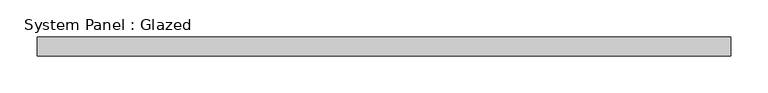
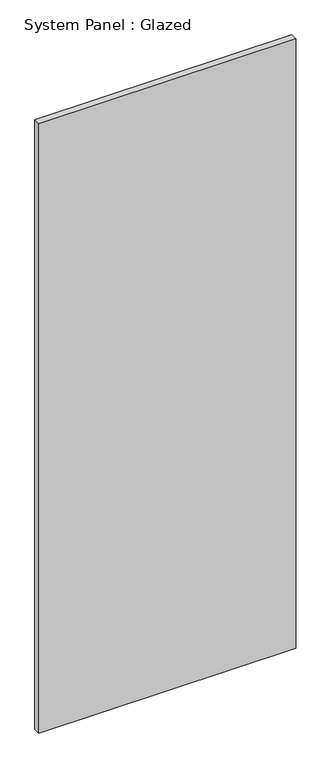
"""IFC4 building model written with IfcOpenShell, lengths in millimetres: plate geometry, System Panel : Glazed."""

from ifc_helpers import new_model, si_unit, origin, origin_with_axes, place, context, project, spatial, polyline, outline, extrude, source, transform, mapped, element, save


def system_panel_glazed_e8343dfa(model_context):
    return source(origin(), model_context, "Body", "SweptSolid", [
        extrude(outline(polyline([(467.0263558, 19.05), (-467.0263558, 19.05), (-467.0263558, 44.45), (467.0263558, 44.45), (467.0263558, 19.05)])), origin_with_axes(), (0.0, 0.0, 1.0), 2343.15),
    ])


if __name__ == "__main__":
    model = new_model("IFC4")
    model_context = context("Model", 3, world=origin())
    ifc_project = project(units=[si_unit("LENGTHUNIT", "METRE", prefix="MILLI")], contexts=[model_context])
    site = spatial("IfcSite", under=ifc_project)
    building = spatial("IfcBuilding", under=site)
    placement = place(None, origin())
    system_panel_glazed_shape = system_panel_glazed_e8343dfa(model_context)
    element("IfcPlate", 1, ObjectType="System Panel : Glazed", at=placement, inside=building, context=model_context, shape_type="MappedRepresentation", body=[
        mapped(system_panel_glazed_shape, transform((0.0, 0.0, 0.0), x_axis=(1.0, 0.0, 0.0), y_axis=(0.0, 1.0, 0.0), z_axis=(0.0, 0.0, 1.0))),
    ])
    save(model, "model.ifc")

# Revit data of these elements
# Type "System Panel : Glazed"
#   Construction Type Id = "GSP4R"
#   Analytic Construction = "1/8 in Pilkington single glazing"
#   Visual Light Transmittance = 0.9
#   Solar Heat Gain Coefficient = 0.86
#   Heat Transfer Coefficient (U) = 1.18115 BTU/(h·ft²·°F)
#   Define Thermal Properties by = 1
# Element 1 (IfcPlate, "System Panel : Glazed")
#   Materials on its faces: "Glass"
# Materials
#   "Glass": class "Glass", colour RGB 0 128 192, transparency 0.75, Description = "Soda Lime Glass", Cost = 0
